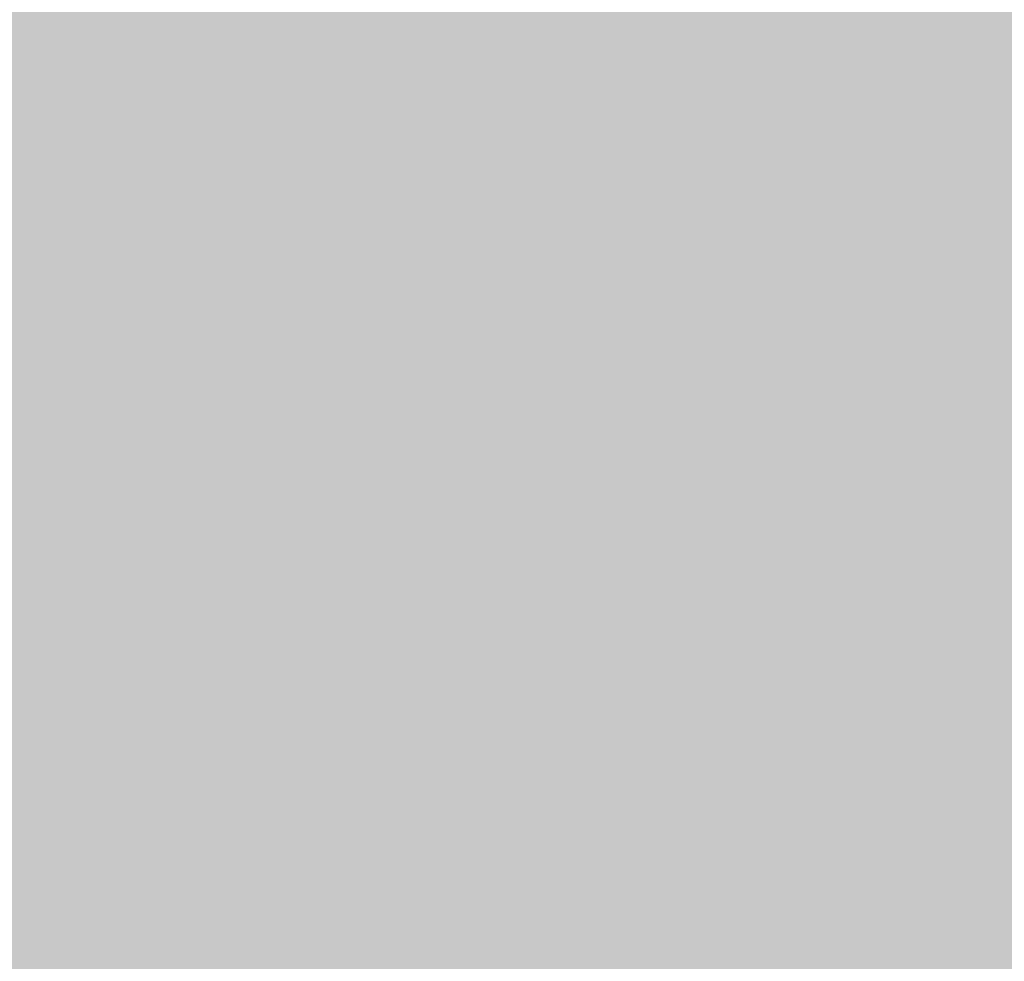
# Model space of a CAD drawing. Units: millimetres. Extents: x 0 to 2267, y 0 to 1823.
# Tile 225 of 256: x 1841.442 to 1842.748, y 1128.399 to 1129.649. Entities that reach past the tile are written whole.
import ezdxf

# ---------------------------------------------------------------- set-up
doc = ezdxf.new("R2010")
doc.units = ezdxf.units.MM
doc.header["$MEASUREMENT"] = 0
doc.layers.add('M-HATC', color=252, linetype='Continuous', lineweight=18)

msp = doc.modelspace()

# ---------------------------------------------------------------- hatches: boundary and pattern name
at = {"layer": 'M-HATC'}
h = msp.add_hatch(color=256, dxfattribs=at)
h.dxf.hatch_style = 1
h.paths.add_polyline_path([(2055.771, 1603.062), (1381.0868, 1603.062), (1381.0868, 1598.062), (2055.771, 1598.062)])
h.paths.add_polyline_path([(2055.771, 1598.062), (1381.0868, 1598.062), (1381.0868, 1593.062), (2055.771, 1593.062)])
h.paths.add_polyline_path([(2051.3074, 1536.7609), (1385.5504, 1536.7609), (1385.5504, 1526.7609), (1387.5504, 1526.7609), (1388.5366, 1525.0528), (1385.3319, 1521.2335), (1385.3319, 1521.2226), (2050.2542, 1522.7491), (2048.3212, 1525.0528), (2049.3074, 1526.7609), (2051.3074, 1526.7609)])
edge = h.paths.add_edge_path()
edge.add_arc((1847.5345, 1379.1492), 135, 222.603061, 222.890851, ccw=False)
edge.add_line((1748.1663, 1287.7656), (1683.0921, 1287.7656))
edge.add_arc((1583.7239, 1379.1492), 135, 317.109149, 317.396939, ccw=False)
edge.add_arc((1678.9686, 1290.6707), 5, 222.8909, 317.1091, ccw=False)
edge.add_arc((1774.2133, 1379.1492), 135, 222.603061, 222.890851, ccw=False)
edge.add_line((1674.8451, 1287.7656), (1609.7709, 1287.7656))
edge.add_arc((1510.4027, 1379.1492), 135, 317.109149, 317.396939, ccw=False)
edge.add_arc((1605.6474, 1290.6707), 5, 222.8909, 317.1091, ccw=False)
edge.add_arc((1700.8921, 1379.1492), 135, 222.603061, 222.890851, ccw=False)
edge.add_line((1601.5239, 1287.7656), (1536.4497, 1287.7656))
edge.add_arc((1437.0815, 1379.1492), 135, 317.109149, 317.396939, ccw=False)
edge.add_arc((1532.3262, 1290.6707), 5, 222.8909, 317.1091, ccw=False)
edge.add_arc((1627.5709, 1379.1492), 135, 222.603061, 222.890851, ccw=False)
edge.add_line((1528.2027, 1287.7656), (1505.9289, 1287.7656))
edge.add_spline(control_points=[(1505.9289, 1287.7656), (1504.2622, 1287.7656), (1504.2622, 1282.7656), (1505.9289, 1282.7656)], knot_values=[0, 0, 0, 0, 5, 5, 5, 5], degree=3, periodic=0)
edge.add_line((1505.9289, 1282.7656), (1930.9289, 1282.7656))
edge.add_spline(control_points=[(1930.9289, 1282.7656), (1932.5956, 1282.7656), (1932.5956, 1287.7656), (1930.9289, 1287.7656)], knot_values=[0, 0, 0, 0, 5, 5, 5, 5], degree=3, periodic=0)
edge.add_line((1930.9289, 1287.7656), (1903.0557, 1287.7656))
edge.add_arc((1803.6875, 1379.1492), 135, 317.109149, 317.396939, ccw=False)
edge.add_arc((1898.9322, 1290.6707), 5, 222.8909, 317.1091, ccw=False)
edge.add_arc((1994.1769, 1379.1492), 135, 222.603061, 222.890851, ccw=False)
edge.add_line((1894.8087, 1287.7656), (1829.7345, 1287.7656))
edge.add_arc((1730.3663, 1379.1492), 135, 317.109149, 317.396939, ccw=False)
edge.add_arc((1825.611, 1290.6707), 5, 222.8909, 317.1091, ccw=False)
edge.add_arc((1920.8557, 1379.1492), 135, 222.603061, 222.890851, ccw=False)
edge.add_line((1821.4875, 1287.7656), (1756.4133, 1287.7656))
edge.add_arc((1657.0451, 1379.1492), 135, 317.109149, 317.396939, ccw=False)
edge.add_arc((1752.2898, 1290.6707), 5, 222.8909, 317.1091, ccw=False)
edge = h.paths.add_edge_path()
edge.add_spline(control_points=[(1843.4289, 1227.2475), (1845.0956, 1227.2475), (1845.0956, 1232.2475), (1843.4289, 1232.2475)], knot_values=[0, 0, 0, 0, 5, 5, 5, 5], degree=3, periodic=0)
edge.add_line((1843.4289, 1232.2475), (1593.4289, 1232.2475))
edge.add_spline(control_points=[(1593.4289, 1232.2475), (1591.7622, 1232.2475), (1591.7622, 1227.2475), (1593.4289, 1227.2475)], knot_values=[0, 0, 0, 0, 5, 5, 5, 5], degree=3, periodic=0)
edge.add_line((1593.4289, 1227.2475), (1843.4289, 1227.2475))
h.paths.add_polyline_path([(1905.9289, 1127.4171), (1530.9289, 1127.4171, 0.414214), (1520.9289, 1117.4171), (1530.9289, 1117.4171), (1915.9289, 1117.4171, 0.414214)])
edge = h.paths.add_edge_path()
edge.add_arc((1397.0858, 1498.4078), 12.7299, 90.78215, 190.87871, ccw=False)
edge.add_line((1396.912, 1511.1365), (1428.0097, 1511.3488))
edge.add_line((1428.0097, 1511.3488), (1433.0097, 1511.3488))
edge.add_line((1433.0097, 1511.3488), (1434.439, 1511.3488))
edge.add_arc((1419.474, 1498.0804), 20, 41.561, 74.08211)
edge.add_line((1424.9592, 1517.3135), (1399.9351, 1517.2561))
edge.add_spline(control_points=[(1399.9307, 1517.2561), (1399.884, 1517.2131), (1399.8328, 1517.1689), (1399.7774, 1517.1236)], knot_values=[11.567499, 11.567499, 11.567499, 11.567499, 11.814249, 11.814249, 11.814249, 11.814249], degree=3, periodic=0)
edge.add_spline(control_points=[(1399.6328, 1517.0099), (1399.5831, 1516.9721), (1399.5307, 1516.9338), (1399.4759, 1516.8947)], knot_values=[11.167718, 11.167718, 11.167718, 11.167718, 11.365188, 11.365188, 11.365188, 11.365188], degree=3, periodic=0)
edge.add_spline(control_points=[(1399.3398, 1516.8001), (1399.1514, 1516.6719), (1398.9384, 1516.5377), (1398.704, 1516.3994)], knot_values=[10.376405, 10.376405, 10.376405, 10.376405, 11.00994, 11.00994, 11.00994, 11.00994], degree=3, periodic=0)
edge.add_spline(control_points=[(1398.6572, 1516.3719), (1398.5789, 1516.326), (1398.4983, 1516.2797), (1398.4155, 1516.2331)], knot_values=[10.125175, 10.125175, 10.125175, 10.125175, 10.334406, 10.334406, 10.334406, 10.334406], degree=3, periodic=0)
edge.add_spline(control_points=[(1398.2642, 1516.1487), (1398.196, 1516.1111), (1398.1263, 1516.0732), (1398.0555, 1516.0351)], knot_values=[9.832246, 9.832246, 9.832246, 9.832246, 9.999658, 9.999658, 9.999658, 9.999658], degree=3, periodic=0)
edge.add_spline(control_points=[(1397.9987, 1516.0048), (1397.7312, 1515.8621), (1397.446, 1515.7171), (1397.1466, 1515.5714)], knot_values=[9.161808, 9.161808, 9.161808, 9.161808, 9.787769, 9.787769, 9.787769, 9.787769], degree=3, periodic=0)
edge.add_spline(control_points=[(1397.1466, 1515.5714), (1396.8418, 1515.423), (1396.5222, 1515.274), (1396.1914, 1515.1262)], knot_values=[8.524455, 8.524455, 8.524455, 8.524455, 9.161808, 9.161808, 9.161808, 9.161808], degree=3, periodic=0)
edge.add_spline(control_points=[(1396.0777, 1515.0756), (1395.9854, 1515.0348), (1395.8922, 1514.994), (1395.7983, 1514.9534)], knot_values=[8.275193, 8.275193, 8.275193, 8.275193, 8.451726, 8.451726, 8.451726, 8.451726], degree=3, periodic=0)
edge.add_spline(control_points=[(1395.6018, 1514.8691), (1395.4997, 1514.8257), (1395.3968, 1514.7824), (1395.2932, 1514.7394)], knot_values=[7.962917, 7.962917, 7.962917, 7.962917, 8.152764, 8.152764, 8.152764, 8.152764], degree=3, periodic=0)
edge.add_spline(control_points=[(1395.2116, 1514.7057), (1394.8278, 1514.5475), (1394.4345, 1514.3929), (1394.0364, 1514.2442)], knot_values=[7.21254, 7.21254, 7.21254, 7.21254, 7.913148, 7.913148, 7.913148, 7.913148], degree=3, periodic=0)
edge.add_spline(control_points=[(1394.0364, 1514.2442), (1393.7076, 1514.1214), (1393.3754, 1514.0027), (1393.0427, 1513.8895)], knot_values=[6.633733, 6.633733, 6.633733, 6.633733, 7.21254, 7.21254, 7.21254, 7.21254], degree=3, periodic=0)
edge.add_spline(control_points=[(1392.8214, 1513.815), (1392.7198, 1513.7812), (1392.6181, 1513.7479), (1392.5166, 1513.7152)], knot_values=[6.328796, 6.328796, 6.328796, 6.328796, 6.505493, 6.505493, 6.505493, 6.505493], degree=3, periodic=0)
edge.add_spline(control_points=[(1392.5166, 1513.7152), (1392.3187, 1513.6515), (1392.1212, 1513.59), (1391.9244, 1513.531)], knot_values=[5.984605, 5.984605, 5.984605, 5.984605, 6.328796, 6.328796, 6.328796, 6.328796], degree=3, periodic=0)
edge.add_spline(control_points=[(1391.7915, 1513.4915), (1391.3122, 1513.3501), (1390.8384, 1513.2239), (1390.3784, 1513.1171)], knot_values=[5.066697, 5.066697, 5.066697, 5.066697, 5.907055, 5.907055, 5.907055, 5.907055], degree=3, periodic=0)
edge.add_spline(control_points=[(1390.3784, 1513.1171), (1390.1797, 1513.071), (1389.9836, 1513.0284), (1389.7907, 1512.9899)], knot_values=[4.70367, 4.70367, 4.70367, 4.70367, 5.066695, 5.066695, 5.066695, 5.066695], degree=3, periodic=0)
edge.add_spline(control_points=[(1389.422, 1512.9204), (1389.2459, 1512.8892), (1389.0729, 1512.8617), (1388.9036, 1512.8381)], knot_values=[4.130571, 4.130571, 4.130571, 4.130571, 4.469816, 4.469816, 4.469816, 4.469816], degree=3, periodic=0)
edge.add_spline(control_points=[(1388.9036, 1512.8381), (1388.591, 1512.7946), (1388.2911, 1512.7644), (1388.0071, 1512.7494)], knot_values=[3.504031, 3.504031, 3.504031, 3.504031, 4.130571, 4.130571, 4.130571, 4.130571], degree=3, periodic=0)
edge.add_spline(control_points=[(1387.9356, 1512.7459), (1387.8538, 1512.7423), (1387.7733, 1512.74), (1387.6944, 1512.739)], knot_values=[3.268866, 3.268866, 3.268866, 3.268866, 3.451164, 3.451164, 3.451164, 3.451164], degree=3, periodic=0)
edge.add_spline(control_points=[(1387.3351, 1512.7443), (1387.2076, 1512.7499), (1387.0847, 1512.7597), (1386.967, 1512.7739)], knot_values=[2.670686, 2.670686, 2.670686, 2.670686, 2.984, 2.984, 2.984, 2.984], degree=3, periodic=0)
edge.add_spline(control_points=[(1386.8327, 1512.7922), (1386.8209, 1512.7941), (1386.8092, 1512.7959), (1386.7975, 1512.7979)], knot_values=[2.516981, 2.516981, 2.516981, 2.516981, 2.549528, 2.549528, 2.549528, 2.549528], degree=3, periodic=0)
edge.add_spline(control_points=[(1386.4526, 1512.8735), (1386.4257, 1512.881), (1386.3993, 1512.889), (1386.3733, 1512.8972)], knot_values=[2.095869, 2.095869, 2.095869, 2.095869, 2.17941, 2.17941, 2.17941, 2.17941], degree=3, periodic=0)
edge.add_spline(control_points=[(1386.0691, 1513.0189), (1386.0634, 1513.0217), (1386.0577, 1513.0246), (1386.052, 1513.0275)], knot_values=[1.72453, 1.72453, 1.72453, 1.72453, 1.745933, 1.745933, 1.745933, 1.745933], degree=3, periodic=0)
edge.add_arc((1399.474, 1498.0804), 20, 131.82432, 180)
edge.add_arc((1630.3336, 1505.5484), 250.9708, 181.705176, 236.427975)
edge.add_arc((1605.3399, 1483.3044), 218.7822, 238.660829, 243.34961)
edge.add_arc((1647.0911, 1510.3592), 262.8986, 183.129836, 237.853442, ccw=False)
h.paths.add_polyline_path([(1406.5369, 1391.9644, 0.149382), (1491.5506, 1296.4418, -0.129517)], flags=17)
edge = h.paths.add_edge_path()
edge.add_arc((2037.3838, 1498.0804), 20, 0, 48.26587)
edge.add_spline(control_points=[(2050.6973, 1513.0052), (2050.6512, 1512.9847), (2050.6034, 1512.9655), (2050.5539, 1512.9477)], knot_values=[1.835652, 1.835652, 1.835652, 1.835652, 2.000781, 2.000781, 2.000781, 2.000781], degree=3, periodic=0)
edge.add_spline(control_points=[(2050.4616, 1512.9166), (2050.479, 1512.9221), (2050.4963, 1512.9277), (2050.5133, 1512.9335)], knot_values=[2.045477, 2.045477, 2.045477, 2.045477, 2.101389, 2.101389, 2.101389, 2.101389], degree=3, periodic=0)
edge.add_spline(control_points=[(2050.129, 1512.8342), (2050.1984, 1512.8473), (2050.2657, 1512.8623), (2050.3308, 1512.8792)], knot_values=[2.237629, 2.237629, 2.237629, 2.237629, 2.435841, 2.435841, 2.435841, 2.435841], degree=3, periodic=0)
edge.add_spline(control_points=[(2050.0946, 1512.8278), (2050.1061, 1512.8299), (2050.1176, 1512.832), (2050.129, 1512.8342)], knot_values=[2.435841, 2.435841, 2.435841, 2.435841, 2.468321, 2.468321, 2.468321, 2.468321], degree=3, periodic=0)
edge.add_spline(control_points=[(2049.7843, 1512.7851), (2049.8552, 1512.7922), (2049.9243, 1512.8008), (2049.9917, 1512.8109)], knot_values=[2.563852, 2.563852, 2.563852, 2.563852, 2.748541, 2.748541, 2.748541, 2.748541], degree=3, periodic=0)
edge.add_spline(control_points=[(2049.4052, 1512.7617), (2049.5364, 1512.7653), (2049.6629, 1512.773), (2049.7843, 1512.7851)], knot_values=[2.748541, 2.748541, 2.748541, 2.748541, 3.064882, 3.064882, 3.064882, 3.064882], degree=3, periodic=0)
edge.add_spline(control_points=[(2049.1698, 1512.7597), (2049.2336, 1512.7591), (2049.2965, 1512.7594), (2049.3584, 1512.7606)], knot_values=[3.102309, 3.102309, 3.102309, 3.102309, 3.2503, 3.2503, 3.2503, 3.2503], degree=3, periodic=0)
edge.add_spline(control_points=[(2048.8573, 1512.7691), (2048.9638, 1512.7638), (2049.068, 1512.7606), (2049.1698, 1512.7597)], knot_values=[3.2503, 3.2503, 3.2503, 3.2503, 3.486069, 3.486069, 3.486069, 3.486069], degree=3, periodic=0)
edge.add_spline(control_points=[(2048.6924, 1512.7789), (2048.3729, 1512.8009), (2048.0345, 1512.8411), (2047.6817, 1512.897)], knot_values=[3.606429, 3.606429, 3.606429, 3.606429, 4.2989, 4.2989, 4.2989, 4.2989], degree=3, periodic=0)
edge.add_spline(control_points=[(2047.6817, 1512.897), (2047.5458, 1512.9185), (2047.4077, 1512.9424), (2047.2678, 1512.9685)], knot_values=[4.2989, 4.2989, 4.2989, 4.2989, 4.565769, 4.565769, 4.565769, 4.565769], degree=3, periodic=0)
edge.add_spline(control_points=[(2047.2678, 1512.9685), (2047.1449, 1512.9914), (2047.0207, 1513.016), (2046.8951, 1513.0422)], knot_values=[4.565769, 4.565769, 4.565769, 4.565769, 4.799971, 4.799971, 4.799971, 4.799971], degree=3, periodic=0)
edge.add_spline(control_points=[(2046.8951, 1513.0422), (2046.5286, 1513.1188), (2046.1513, 1513.209), (2045.7676, 1513.3107)], knot_values=[4.799971, 4.799971, 4.799971, 4.799971, 5.483718, 5.483718, 5.483718, 5.483718], degree=3, periodic=0)
edge.add_spline(control_points=[(2045.7676, 1513.3107), (2045.3724, 1513.4154), (2044.9704, 1513.5322), (2044.5662, 1513.6588)], knot_values=[5.483718, 5.483718, 5.483718, 5.483718, 6.187866, 6.187866, 6.187866, 6.187866], degree=3, periodic=0)
edge.add_spline(control_points=[(2044.5662, 1513.6588), (2044.4149, 1513.7061), (2044.2633, 1513.7549), (2044.1116, 1513.8048)], knot_values=[6.187866, 6.187866, 6.187866, 6.187866, 6.451551, 6.451551, 6.451551, 6.451551], degree=3, periodic=0)
edge.add_spline(control_points=[(2044.1116, 1513.8048), (2043.9967, 1513.8427), (2043.8817, 1513.8813), (2043.7668, 1513.9205)], knot_values=[6.451551, 6.451551, 6.451551, 6.451551, 6.651434, 6.651434, 6.651434, 6.651434], degree=3, periodic=0)
edge.add_spline(control_points=[(2043.7668, 1513.9205), (2043.3716, 1514.0554), (2042.9774, 1514.1979), (2042.5886, 1514.3458)], knot_values=[6.651434, 6.651434, 6.651434, 6.651434, 7.338879, 7.338879, 7.338879, 7.338879], degree=3, periodic=0)
edge.add_spline(control_points=[(2042.5886, 1514.3458), (2042.1643, 1514.5071), (2041.7465, 1514.6749), (2041.3409, 1514.846)], knot_values=[7.338879, 7.338879, 7.338879, 7.338879, 8.089209, 8.089209, 8.089209, 8.089209], degree=3, periodic=0)
edge.add_spline(control_points=[(2041.3409, 1514.846), (2041.1028, 1514.9465), (2040.869, 1515.0481), (2040.6405, 1515.1502)], knot_values=[8.089209, 8.089209, 8.089209, 8.089209, 8.529587, 8.529587, 8.529587, 8.529587], degree=3, periodic=0)
edge.add_spline(control_points=[(2040.51, 1515.2089), (2040.0824, 1515.4022), (2039.6747, 1515.5971), (2039.295, 1515.7894)], knot_values=[8.613818, 8.613818, 8.613818, 8.613818, 9.44571, 9.44571, 9.44571, 9.44571], degree=3, periodic=0)
edge.add_spline(control_points=[(2039.295, 1515.7894), (2039.0618, 1515.9075), (2038.8391, 1516.0246), (2038.6288, 1516.1398)], knot_values=[9.44571, 9.44571, 9.44571, 9.44571, 9.956404, 9.956404, 9.956404, 9.956404], degree=3, periodic=0)
edge.add_spline(control_points=[(2038.6288, 1516.1398), (2038.5187, 1516.2001), (2038.4121, 1516.2598), (2038.309, 1516.3189)], knot_values=[9.956404, 9.956404, 9.956404, 9.956404, 10.223542, 10.223542, 10.223542, 10.223542], degree=3, periodic=0)
edge.add_spline(control_points=[(2038.309, 1516.3189), (2038.2138, 1516.3735), (2038.1216, 1516.4276), (2038.0328, 1516.481)], knot_values=[10.223542, 10.223542, 10.223542, 10.223542, 10.47051, 10.47051, 10.47051, 10.47051], degree=3, periodic=0)
edge.add_spline(control_points=[(2038.0328, 1516.481), (2037.7855, 1516.6296), (2037.5639, 1516.773), (2037.3722, 1516.909)], knot_values=[10.47051, 10.47051, 10.47051, 10.47051, 11.15767, 11.15767, 11.15767, 11.15767], degree=3, periodic=0)
edge.add_spline(control_points=[(2037.3722, 1516.909), (2037.2789, 1516.9752), (2037.1927, 1517.0396), (2037.1142, 1517.102)], knot_values=[11.15767, 11.15767, 11.15767, 11.15767, 11.49227, 11.49227, 11.49227, 11.49227], degree=3, periodic=0)
edge.add_spline(control_points=[(2036.8564, 1517.3259), (2036.9148, 1517.2692), (2036.9814, 1517.2103), (2037.0557, 1517.1492)], knot_values=[11.577341, 11.577341, 11.577341, 11.577341, 11.91035, 11.91035, 11.91035, 11.91035], degree=3, periodic=0)
edge.add_spline(control_points=[(2036.8074, 1517.3748), (2036.823, 1517.3587), (2036.8393, 1517.3424), (2036.8564, 1517.3259)], knot_values=[11.91035, 11.91035, 11.91035, 11.91035, 12.007402, 12.007402, 12.007402, 12.007402], degree=3, periodic=0)
edge.add_spline(control_points=[(2036.7017, 1517.494), (2036.7104, 1517.483), (2036.7196, 1517.4719), (2036.7291, 1517.4606)], knot_values=[12.184155, 12.184155, 12.184155, 12.184155, 12.255409, 12.255409, 12.255409, 12.255409], degree=3, periodic=0)
edge.add_spline(control_points=[(2036.6159, 1517.6205), (2036.62, 1517.613), (2036.6243, 1517.6055), (2036.6289, 1517.5979)], knot_values=[12.487913, 12.487913, 12.487913, 12.487913, 12.541035, 12.541035, 12.541035, 12.541035], degree=3, periodic=0)
edge.add_spline(control_points=[(2036.5635, 1517.786), (2036.5637, 1517.7794), (2036.5642, 1517.7726), (2036.565, 1517.7658)], knot_values=[12.911761, 12.911761, 12.911761, 12.911761, 12.968286, 12.968286, 12.968286, 12.968286], degree=3, periodic=0)
edge.add_spline(control_points=[(2036.6166, 1517.9304), (2036.6125, 1517.9259), (2036.6086, 1517.9212), (2036.6049, 1517.9165)], knot_values=[13.382527, 13.382527, 13.382527, 13.382527, 13.433791, 13.433791, 13.433791, 13.433791], degree=3, periodic=0)
edge.add_spline(control_points=[(2036.749, 1518.017), (2036.7361, 1518.0116), (2036.7239, 1518.006), (2036.7124, 1518.0002)], knot_values=[13.726299, 13.726299, 13.726299, 13.726299, 13.809928, 13.809928, 13.809928, 13.809928], degree=3, periodic=0)
edge.add_spline(control_points=[(2036.8604, 1518.0528), (2036.8386, 1518.0474), (2036.8181, 1518.0416), (2036.7988, 1518.0353)], knot_values=[13.910887, 13.910887, 13.910887, 13.910887, 14.02153, 14.02153, 14.02153, 14.02153], degree=3, periodic=0)
edge.add_line((2036.9639, 1518.0804), (2032.3838, 1518.0804))
edge.add_line((2032.3838, 1518.0804), (2027.3838, 1518.0804))
edge.add_line((2027.3838, 1518.0804), (2022.3838, 1518.0804))
edge.add_line((2022.3838, 1518.0804), (2017.3838, 1518.0804))
edge.add_arc((2017.3838, 1498.0804), 20, 90, 138.439)
edge.add_line((2002.4188, 1511.3488), (2003.8481, 1511.3488))
edge.add_line((2003.8481, 1511.3488), (2008.8481, 1511.3488))
edge.add_line((2008.8481, 1511.3488), (2039.772, 1511.1377))
edge.add_arc((2039.772, 1498.4078), 12.7299, -10.87871, 90, ccw=False)
edge.add_arc((1789.7668, 1510.3592), 262.8986, 302.146558, 356.870164, ccw=False)
edge.add_arc((1831.5179, 1483.3044), 218.7822, 296.65039, 301.339171)
edge.add_arc((1806.5242, 1505.5484), 250.9708, 303.572025, 358.294824)
h.paths.add_polyline_path([(2030.321, 1391.9644, -0.129517), (1945.3072, 1296.4418, 0.149382)], flags=17)
edge = h.paths.add_edge_path()
edge.add_spline(control_points=[(2037.2464, 1518.0821), (2037.2898, 1518.081), (2037.3355, 1518.0804), (2037.3838, 1518.0804)], knot_values=[0.000012, 0.000012, 0.000012, 0.000012, 0.144754, 0.144754, 0.144754, 0.144754], degree=3, periodic=0)
edge.add_line((2037.3357, 1518.0804), (2037.0096, 1518.0804))
edge.add_spline(control_points=[(2037.0096, 1518.0804), (2036.9822, 1518.0768), (2036.956, 1518.0727), (2036.9312, 1518.0681)], knot_values=[14.13465, 14.13465, 14.13465, 14.13465, 14.247197, 14.247197, 14.247197, 14.247197], degree=3, periodic=0)
edge.add_spline(control_points=[(2036.9312, 1518.0681), (2036.9276, 1518.0674), (2036.9241, 1518.0667), (2036.9205, 1518.0661)], knot_values=[14.118315, 14.118315, 14.118315, 14.118315, 14.13465, 14.13465, 14.13465, 14.13465], degree=3, periodic=0)
edge.add_spline(control_points=[(2036.9205, 1518.0661), (2036.9118, 1518.0644), (2036.9032, 1518.0626), (2036.8948, 1518.0608)], knot_values=[14.078086, 14.078086, 14.078086, 14.078086, 14.118315, 14.118315, 14.118315, 14.118315], degree=3, periodic=0)
edge.add_spline(control_points=[(2036.8948, 1518.0608), (2036.883, 1518.0583), (2036.8716, 1518.0556), (2036.8604, 1518.0528)], knot_values=[14.02153, 14.02153, 14.02153, 14.02153, 14.078086, 14.078086, 14.078086, 14.078086], degree=3, periodic=0)
edge.add_spline(control_points=[(2036.8604, 1518.0528), (2036.8386, 1518.0474), (2036.8181, 1518.0416), (2036.7988, 1518.0353)], knot_values=[13.910887, 13.910887, 13.910887, 13.910887, 14.02153, 14.02153, 14.02153, 14.02153], degree=3, periodic=0)
edge.add_spline(control_points=[(2036.7988, 1518.0353), (2036.7981, 1518.035), (2036.7974, 1518.0348), (2036.7967, 1518.0346)], knot_values=[13.906906, 13.906906, 13.906906, 13.906906, 13.910887, 13.910887, 13.910887, 13.910887], degree=3, periodic=0)
edge.add_spline(control_points=[(2036.7967, 1518.0346), (2036.7882, 1518.0318), (2036.7799, 1518.0289), (2036.7719, 1518.0259)], knot_values=[13.857826, 13.857826, 13.857826, 13.857826, 13.906906, 13.906906, 13.906906, 13.906906], degree=3, periodic=0)
edge.add_spline(control_points=[(2036.7719, 1518.0259), (2036.764, 1518.023), (2036.7564, 1518.02), (2036.749, 1518.017)], knot_values=[13.809928, 13.809928, 13.809928, 13.809928, 13.857826, 13.857826, 13.857826, 13.857826], degree=3, periodic=0)
edge.add_spline(control_points=[(2036.749, 1518.017), (2036.7361, 1518.0116), (2036.7239, 1518.006), (2036.7124, 1518.0002)], knot_values=[13.726299, 13.726299, 13.726299, 13.726299, 13.809928, 13.809928, 13.809928, 13.809928], degree=3, periodic=0)
edge.add_spline(control_points=[(2036.7124, 1518.0002), (2036.7121, 1518), (2036.7118, 1517.9999), (2036.7115, 1517.9997)], knot_values=[13.723993, 13.723993, 13.723993, 13.723993, 13.726299, 13.726299, 13.726299, 13.726299], degree=3, periodic=0)
edge.add_spline(control_points=[(2036.7115, 1517.9997), (2036.7063, 1517.9971), (2036.7013, 1517.9944), (2036.6965, 1517.9917)], knot_values=[13.686536, 13.686536, 13.686536, 13.686536, 13.723993, 13.723993, 13.723993, 13.723993], degree=3, periodic=0)
edge.add_spline(control_points=[(2036.6965, 1517.9917), (2036.6919, 1517.9891), (2036.6874, 1517.9865), (2036.6831, 1517.9839)], knot_values=[13.651251, 13.651251, 13.651251, 13.651251, 13.686536, 13.686536, 13.686536, 13.686536], degree=3, periodic=0)
edge.add_spline(control_points=[(2036.6831, 1517.9839), (2036.6764, 1517.9798), (2036.67, 1517.9757), (2036.6639, 1517.9714)], knot_values=[13.596804, 13.596804, 13.596804, 13.596804, 13.651251, 13.651251, 13.651251, 13.651251], degree=3, periodic=0)
edge.add_spline(control_points=[(2036.6639, 1517.9714), (2036.6636, 1517.9712), (2036.6633, 1517.9709), (2036.6629, 1517.9707)], knot_values=[13.593956, 13.593956, 13.593956, 13.593956, 13.596804, 13.596804, 13.596804, 13.596804], degree=3, periodic=0)
edge.add_spline(control_points=[(2036.6629, 1517.9707), (2036.6603, 1517.9689), (2036.6577, 1517.967), (2036.6552, 1517.9651)], knot_values=[13.570322, 13.570322, 13.570322, 13.570322, 13.593956, 13.593956, 13.593956, 13.593956], degree=3, periodic=0)
edge.add_spline(control_points=[(2036.6552, 1517.9651), (2036.6525, 1517.9631), (2036.6499, 1517.9611), (2036.6474, 1517.9591)], knot_values=[13.545477, 13.545477, 13.545477, 13.545477, 13.570322, 13.570322, 13.570322, 13.570322], degree=3, periodic=0)
edge.add_spline(control_points=[(2036.6474, 1517.9591), (2036.6472, 1517.9589), (2036.6471, 1517.9588), (2036.6469, 1517.9587)], knot_values=[13.543931, 13.543931, 13.543931, 13.543931, 13.545477, 13.545477, 13.545477, 13.545477], degree=3, periodic=0)
edge.add_spline(control_points=[(2036.6469, 1517.9587), (2036.6412, 1517.9541), (2036.6358, 1517.9494), (2036.6307, 1517.9447)], knot_values=[13.488237, 13.488237, 13.488237, 13.488237, 13.543931, 13.543931, 13.543931, 13.543931], degree=3, periodic=0)
edge.add_spline(control_points=[(2036.6307, 1517.9447), (2036.6282, 1517.9423), (2036.6257, 1517.9399), (2036.6233, 1517.9374)], knot_values=[13.460307, 13.460307, 13.460307, 13.460307, 13.488237, 13.488237, 13.488237, 13.488237], degree=3, periodic=0)
edge.add_spline(control_points=[(2036.6233, 1517.9374), (2036.6215, 1517.9356), (2036.6198, 1517.9338), (2036.6181, 1517.932)], knot_values=[13.439712, 13.439712, 13.439712, 13.439712, 13.460307, 13.460307, 13.460307, 13.460307], degree=3, periodic=0)
edge.add_spline(control_points=[(2036.6181, 1517.932), (2036.6176, 1517.9315), (2036.6171, 1517.9309), (2036.6166, 1517.9304)], knot_values=[13.433791, 13.433791, 13.433791, 13.433791, 13.439712, 13.439712, 13.439712, 13.439712], degree=3, periodic=0)
edge.add_spline(control_points=[(2036.6166, 1517.9304), (2036.6125, 1517.9259), (2036.6086, 1517.9212), (2036.6049, 1517.9165)], knot_values=[13.382527, 13.382527, 13.382527, 13.382527, 13.433791, 13.433791, 13.433791, 13.433791], degree=3, periodic=0)
edge.add_spline(control_points=[(2036.6049, 1517.9165), (2036.6026, 1517.9135), (2036.6004, 1517.9104), (2036.5982, 1517.9074)], knot_values=[13.350017, 13.350017, 13.350017, 13.350017, 13.382527, 13.382527, 13.382527, 13.382527], degree=3, periodic=0)
edge.add_spline(control_points=[(2036.5982, 1517.9074), (2036.5972, 1517.9059), (2036.5962, 1517.9043), (2036.5952, 1517.9028)], knot_values=[13.333922, 13.333922, 13.333922, 13.333922, 13.350017, 13.350017, 13.350017, 13.350017], degree=3, periodic=0)
edge.add_spline(control_points=[(2036.5952, 1517.9028), (2036.5945, 1517.9018), (2036.5939, 1517.9009), (2036.5933, 1517.8999)], knot_values=[13.323828, 13.323828, 13.323828, 13.323828, 13.333922, 13.333922, 13.333922, 13.333922], degree=3, periodic=0)
edge.add_spline(control_points=[(2036.5933, 1517.8999), (2036.5905, 1517.8955), (2036.5879, 1517.8909), (2036.5855, 1517.8864)], knot_values=[13.277545, 13.277545, 13.277545, 13.277545, 13.323828, 13.323828, 13.323828, 13.323828], degree=3, periodic=0)
edge.add_spline(control_points=[(2036.5855, 1517.8864), (2036.5836, 1517.8827), (2036.5817, 1517.8789), (2036.5801, 1517.8751)], knot_values=[13.240119, 13.240119, 13.240119, 13.240119, 13.277545, 13.277545, 13.277545, 13.277545], degree=3, periodic=0)
edge.add_spline(control_points=[(2036.5801, 1517.8751), (2036.5795, 1517.8739), (2036.579, 1517.8727), (2036.5785, 1517.8715)], knot_values=[13.228211, 13.228211, 13.228211, 13.228211, 13.240119, 13.240119, 13.240119, 13.240119], degree=3, periodic=0)
edge.add_spline(control_points=[(2036.5785, 1517.8715), (2036.578, 1517.8702), (2036.5774, 1517.869), (2036.5769, 1517.8677)], knot_values=[13.215717, 13.215717, 13.215717, 13.215717, 13.228211, 13.228211, 13.228211, 13.228211], degree=3, periodic=0)
edge.add_spline(control_points=[(2036.5769, 1517.8677), (2036.5755, 1517.864), (2036.5741, 1517.8603), (2036.5729, 1517.8565)], knot_values=[13.179847, 13.179847, 13.179847, 13.179847, 13.215717, 13.215717, 13.215717, 13.215717], degree=3, periodic=0)
edge.add_spline(control_points=[(2036.5729, 1517.8565), (2036.5713, 1517.8515), (2036.5699, 1517.8464), (2036.5687, 1517.8413)], knot_values=[13.132017, 13.132017, 13.132017, 13.132017, 13.179847, 13.179847, 13.179847, 13.179847], degree=3, periodic=0)
edge.add_spline(control_points=[(2036.5687, 1517.8413), (2036.5684, 1517.8402), (2036.5682, 1517.8392), (2036.568, 1517.8382)], knot_values=[13.122482, 13.122482, 13.122482, 13.122482, 13.132017, 13.132017, 13.132017, 13.132017], degree=3, periodic=0)
edge.add_spline(control_points=[(2036.568, 1517.8382), (2036.5676, 1517.8363), (2036.5672, 1517.8345), (2036.5669, 1517.8327)], knot_values=[13.105592, 13.105592, 13.105592, 13.105592, 13.122482, 13.122482, 13.122482, 13.122482], degree=3, periodic=0)
edge.add_spline(control_points=[(2036.5669, 1517.8327), (2036.5662, 1517.8292), (2036.5657, 1517.8257), (2036.5652, 1517.8222)], knot_values=[13.074063, 13.074063, 13.074063, 13.074063, 13.105592, 13.105592, 13.105592, 13.105592], degree=3, periodic=0)
edge.add_spline(control_points=[(2036.5652, 1517.8222), (2036.5652, 1517.8222), (2036.5652, 1517.8222), (2036.5652, 1517.8222)], knot_values=[13.074043, 13.074043, 13.074043, 13.074043, 13.074063, 13.074063, 13.074063, 13.074063], degree=3, periodic=0)
edge.add_spline(control_points=[(2036.5652, 1517.8222), (2036.5644, 1517.8164), (2036.5639, 1517.8106), (2036.5636, 1517.8046)], knot_values=[13.021884, 13.021884, 13.021884, 13.021884, 13.074043, 13.074043, 13.074043, 13.074043], degree=3, periodic=0)
edge.add_spline(control_points=[(2036.5636, 1517.8046), (2036.5636, 1517.804), (2036.5636, 1517.8034), (2036.5635, 1517.8028)], knot_values=[13.01674, 13.01674, 13.01674, 13.01674, 13.021884, 13.021884, 13.021884, 13.021884], degree=3, periodic=0)
edge.add_spline(control_points=[(2036.5635, 1517.8028), (2036.5634, 1517.8005), (2036.5634, 1517.7982), (2036.5634, 1517.7958)], knot_values=[12.996438, 12.996438, 12.996438, 12.996438, 13.01674, 13.01674, 13.01674, 13.01674], degree=3, periodic=0)
edge.add_spline(control_points=[(2036.5634, 1517.7958), (2036.5633, 1517.7926), (2036.5634, 1517.7893), (2036.5635, 1517.786)], knot_values=[12.968286, 12.968286, 12.968286, 12.968286, 12.996438, 12.996438, 12.996438, 12.996438], degree=3, periodic=0)
edge.add_spline(control_points=[(2036.5635, 1517.786), (2036.5637, 1517.7794), (2036.5642, 1517.7726), (2036.565, 1517.7658)], knot_values=[12.911761, 12.911761, 12.911761, 12.911761, 12.968286, 12.968286, 12.968286, 12.968286], degree=3, periodic=0)
edge.add_spline(control_points=[(2036.565, 1517.7658), (2036.565, 1517.7657), (2036.565, 1517.7656), (2036.565, 1517.7656)], knot_values=[12.911017, 12.911017, 12.911017, 12.911017, 12.911761, 12.911761, 12.911761, 12.911761], degree=3, periodic=0)
edge.add_spline(control_points=[(2036.565, 1517.7656), (2036.5654, 1517.7625), (2036.5658, 1517.7593), (2036.5663, 1517.7562)], knot_values=[12.88528, 12.88528, 12.88528, 12.88528, 12.911017, 12.911017, 12.911017, 12.911017], degree=3, periodic=0)
edge.add_spline(control_points=[(2036.5663, 1517.7562), (2036.5667, 1517.7534), (2036.5672, 1517.7506), (2036.5677, 1517.7478)], knot_values=[12.862519, 12.862519, 12.862519, 12.862519, 12.88528, 12.88528, 12.88528, 12.88528], degree=3, periodic=0)
edge.add_spline(control_points=[(2036.5677, 1517.7478), (2036.5678, 1517.7474), (2036.5679, 1517.7469), (2036.568, 1517.7465)], knot_values=[12.858885, 12.858885, 12.858885, 12.858885, 12.862519, 12.862519, 12.862519, 12.862519], degree=3, periodic=0)
edge.add_spline(control_points=[(2036.568, 1517.7465), (2036.5692, 1517.7399), (2036.5707, 1517.7332), (2036.5724, 1517.7264)], knot_values=[12.8053, 12.8053, 12.8053, 12.8053, 12.858885, 12.858885, 12.858885, 12.858885], degree=3, periodic=0)
edge.add_spline(control_points=[(2036.5724, 1517.7264), (2036.5734, 1517.7226), (2036.5745, 1517.7187), (2036.5756, 1517.7149)], knot_values=[12.775176, 12.775176, 12.775176, 12.775176, 12.8053, 12.8053, 12.8053, 12.8053], degree=3, periodic=0)
edge.add_spline(control_points=[(2036.5756, 1517.7149), (2036.5763, 1517.7125), (2036.577, 1517.7102), (2036.5778, 1517.7078)], knot_values=[12.756759, 12.756759, 12.756759, 12.756759, 12.775176, 12.775176, 12.775176, 12.775176], degree=3, periodic=0)
edge.add_spline(control_points=[(2036.5778, 1517.7078), (2036.5781, 1517.7067), (2036.5784, 1517.7057), (2036.5787, 1517.7047)], knot_values=[12.748742, 12.748742, 12.748742, 12.748742, 12.756759, 12.756759, 12.756759, 12.756759], degree=3, periodic=0)
edge.add_spline(control_points=[(2036.5787, 1517.7047), (2036.5808, 1517.6983), (2036.5831, 1517.6919), (2036.5856, 1517.6854)], knot_values=[12.69959, 12.69959, 12.69959, 12.69959, 12.748742, 12.748742, 12.748742, 12.748742], degree=3, periodic=0)
edge.add_spline(control_points=[(2036.5856, 1517.6854), (2036.5876, 1517.68), (2036.5898, 1517.6746), (2036.5921, 1517.6692)], knot_values=[12.659038, 12.659038, 12.659038, 12.659038, 12.69959, 12.69959, 12.69959, 12.69959], degree=3, periodic=0)
edge.add_spline(control_points=[(2036.5921, 1517.6692), (2036.594, 1517.6648), (2036.5959, 1517.6605), (2036.5979, 1517.6561)], knot_values=[12.626806, 12.626806, 12.626806, 12.626806, 12.659038, 12.659038, 12.659038, 12.659038], degree=3, periodic=0)
edge.add_spline(control_points=[(2036.5979, 1517.6561), (2036.5984, 1517.6551), (2036.5989, 1517.6541), (2036.5993, 1517.6531)], knot_values=[12.619394, 12.619394, 12.619394, 12.619394, 12.626806, 12.626806, 12.626806, 12.626806], degree=3, periodic=0)
edge.add_spline(control_points=[(2036.5993, 1517.6531), (2036.6043, 1517.6424), (2036.6099, 1517.6315), (2036.6159, 1517.6205)], knot_values=[12.541039, 12.541039, 12.541039, 12.541039, 12.619394, 12.619394, 12.619394, 12.619394], degree=3, periodic=0)
edge.add_spline(control_points=[(2036.6159, 1517.6205), (2036.6159, 1517.6205), (2036.6159, 1517.6205), (2036.6159, 1517.6205)], knot_values=[12.541035, 12.541035, 12.541035, 12.541035, 12.541039, 12.541039, 12.541039, 12.541039], degree=3, periodic=0)
edge.add_spline(control_points=[(2036.6159, 1517.6205), (2036.62, 1517.613), (2036.6243, 1517.6055), (2036.6289, 1517.5979)], knot_values=[12.487913, 12.487913, 12.487913, 12.487913, 12.541035, 12.541035, 12.541035, 12.541035], degree=3, periodic=0)
edge.add_spline(control_points=[(2036.6289, 1517.5979), (2036.6326, 1517.5916), (2036.6365, 1517.5853), (2036.6406, 1517.5789)], knot_values=[12.443982, 12.443982, 12.443982, 12.443982, 12.487913, 12.487913, 12.487913, 12.487913], degree=3, periodic=0)
edge.add_spline(control_points=[(2036.6406, 1517.5789), (2036.6414, 1517.5776), (2036.6423, 1517.5763), (2036.6431, 1517.5749)], knot_values=[12.434996, 12.434996, 12.434996, 12.434996, 12.443982, 12.443982, 12.443982, 12.443982], degree=3, periodic=0)
edge.add_spline(control_points=[(2036.6431, 1517.5749), (2036.6531, 1517.5596), (2036.6639, 1517.5439), (2036.6756, 1517.528)], knot_values=[12.329647, 12.329647, 12.329647, 12.329647, 12.434996, 12.434996, 12.434996, 12.434996], degree=3, periodic=0)
edge.add_spline(control_points=[(2036.6756, 1517.528), (2036.6839, 1517.5168), (2036.6925, 1517.5055), (2036.7017, 1517.494)], knot_values=[12.255409, 12.255409, 12.255409, 12.255409, 12.329647, 12.329647, 12.329647, 12.329647], degree=3, periodic=0)
edge.add_spline(control_points=[(2036.7017, 1517.494), (2036.7104, 1517.483), (2036.7196, 1517.4719), (2036.7291, 1517.4606)], knot_values=[12.184155, 12.184155, 12.184155, 12.184155, 12.255409, 12.255409, 12.255409, 12.255409], degree=3, periodic=0)
edge.add_spline(control_points=[(2036.7291, 1517.4606), (2036.7436, 1517.4435), (2036.759, 1517.4262), (2036.7753, 1517.4085)], knot_values=[12.075961, 12.075961, 12.075961, 12.075961, 12.184155, 12.184155, 12.184155, 12.184155], degree=3, periodic=0)
edge.add_spline(control_points=[(2036.7753, 1517.4085), (2036.7763, 1517.4075), (2036.7773, 1517.4064), (2036.7783, 1517.4054)], knot_values=[12.069502, 12.069502, 12.069502, 12.069502, 12.075961, 12.075961, 12.075961, 12.075961], degree=3, periodic=0)
edge.add_spline(control_points=[(2036.7783, 1517.4054), (2036.7877, 1517.3953), (2036.7974, 1517.385), (2036.8074, 1517.3748)], knot_values=[12.007402, 12.007402, 12.007402, 12.007402, 12.069502, 12.069502, 12.069502, 12.069502], degree=3, periodic=0)
edge.add_spline(control_points=[(2036.8074, 1517.3748), (2036.823, 1517.3587), (2036.8393, 1517.3424), (2036.8564, 1517.3259)], knot_values=[11.91035, 11.91035, 11.91035, 11.91035, 12.007402, 12.007402, 12.007402, 12.007402], degree=3, periodic=0)
edge.add_spline(control_points=[(2036.8564, 1517.3259), (2036.9148, 1517.2692), (2036.9814, 1517.2103), (2037.0557, 1517.1492)], knot_values=[11.577341, 11.577341, 11.577341, 11.577341, 11.91035, 11.91035, 11.91035, 11.91035], degree=3, periodic=0)
edge.add_spline(control_points=[(2037.0557, 1517.1492), (2037.0747, 1517.1336), (2037.0942, 1517.1179), (2037.1142, 1517.102)], knot_values=[11.49227, 11.49227, 11.49227, 11.49227, 11.577341, 11.577341, 11.577341, 11.577341], degree=3, periodic=0)
edge.add_spline(control_points=[(2037.1142, 1517.102), (2037.1927, 1517.0396), (2037.2789, 1516.9752), (2037.3722, 1516.909)], knot_values=[11.15767, 11.15767, 11.15767, 11.15767, 11.49227, 11.49227, 11.49227, 11.49227], degree=3, periodic=0)
edge.add_spline(control_points=[(2037.3722, 1516.909), (2037.5639, 1516.773), (2037.7855, 1516.6296), (2038.0328, 1516.481)], knot_values=[10.47051, 10.47051, 10.47051, 10.47051, 11.15767, 11.15767, 11.15767, 11.15767], degree=3, periodic=0)
edge.add_spline(control_points=[(2038.0328, 1516.481), (2038.1216, 1516.4276), (2038.2138, 1516.3735), (2038.309, 1516.3189)], knot_values=[10.223542, 10.223542, 10.223542, 10.223542, 10.47051, 10.47051, 10.47051, 10.47051], degree=3, periodic=0)
edge.add_spline(control_points=[(2038.309, 1516.3189), (2038.4121, 1516.2598), (2038.5187, 1516.2001), (2038.6288, 1516.1398)], knot_values=[9.956404, 9.956404, 9.956404, 9.956404, 10.223542, 10.223542, 10.223542, 10.223542], degree=3, periodic=0)
edge.add_spline(control_points=[(2038.6288, 1516.1398), (2038.8391, 1516.0246), (2039.0618, 1515.9075), (2039.295, 1515.7894)], knot_values=[9.44571, 9.44571, 9.44571, 9.44571, 9.956404, 9.956404, 9.956404, 9.956404], degree=3, periodic=0)
edge.add_spline(control_points=[(2039.295, 1515.7894), (2039.6747, 1515.5971), (2040.0824, 1515.4022), (2040.51, 1515.2089)], knot_values=[8.613818, 8.613818, 8.613818, 8.613818, 9.44571, 9.44571, 9.44571, 9.44571], degree=3, periodic=0)
edge.add_spline(control_points=[(2040.51, 1515.2089), (2040.5533, 1515.1893), (2040.5968, 1515.1697), (2040.6405, 1515.1502)], knot_values=[8.529587, 8.529587, 8.529587, 8.529587, 8.613818, 8.613818, 8.613818, 8.613818], degree=3, periodic=0)
edge.add_spline(control_points=[(2040.6405, 1515.1502), (2040.869, 1515.0481), (2041.1028, 1514.9465), (2041.3409, 1514.846)], knot_values=[8.089209, 8.089209, 8.089209, 8.089209, 8.529587, 8.529587, 8.529587, 8.529587], degree=3, periodic=0)
edge.add_spline(control_points=[(2041.3409, 1514.846), (2041.7465, 1514.6749), (2042.1643, 1514.5071), (2042.5886, 1514.3458)], knot_values=[7.338879, 7.338879, 7.338879, 7.338879, 8.089209, 8.089209, 8.089209, 8.089209], degree=3, periodic=0)
edge.add_spline(control_points=[(2042.5886, 1514.3458), (2042.9774, 1514.1979), (2043.3716, 1514.0554), (2043.7668, 1513.9205)], knot_values=[6.651434, 6.651434, 6.651434, 6.651434, 7.338879, 7.338879, 7.338879, 7.338879], degree=3, periodic=0)
edge.add_spline(control_points=[(2043.7668, 1513.9205), (2043.8817, 1513.8813), (2043.9967, 1513.8427), (2044.1116, 1513.8048)], knot_values=[6.451551, 6.451551, 6.451551, 6.451551, 6.651434, 6.651434, 6.651434, 6.651434], degree=3, periodic=0)
edge.add_spline(control_points=[(2044.1116, 1513.8048), (2044.2633, 1513.7549), (2044.4149, 1513.7061), (2044.5662, 1513.6588)], knot_values=[6.187866, 6.187866, 6.187866, 6.187866, 6.451551, 6.451551, 6.451551, 6.451551], degree=3, periodic=0)
edge.add_spline(control_points=[(2044.5662, 1513.6588), (2044.9704, 1513.5322), (2045.3724, 1513.4154), (2045.7676, 1513.3107)], knot_values=[5.483718, 5.483718, 5.483718, 5.483718, 6.187866, 6.187866, 6.187866, 6.187866], degree=3, periodic=0)
edge.add_spline(control_points=[(2045.7676, 1513.3107), (2046.1513, 1513.209), (2046.5286, 1513.1188), (2046.8951, 1513.0422)], knot_values=[4.799971, 4.799971, 4.799971, 4.799971, 5.483718, 5.483718, 5.483718, 5.483718], degree=3, periodic=0)
edge.add_spline(control_points=[(2046.8951, 1513.0422), (2047.0207, 1513.016), (2047.1449, 1512.9914), (2047.2678, 1512.9685)], knot_values=[4.565769, 4.565769, 4.565769, 4.565769, 4.799971, 4.799971, 4.799971, 4.799971], degree=3, periodic=0)
edge.add_spline(control_points=[(2047.2678, 1512.9685), (2047.4077, 1512.9424), (2047.5458, 1512.9185), (2047.6817, 1512.897)], knot_values=[4.2989, 4.2989, 4.2989, 4.2989, 4.565769, 4.565769, 4.565769, 4.565769], degree=3, periodic=0)
edge.add_spline(control_points=[(2047.6817, 1512.897), (2048.0345, 1512.8411), (2048.3729, 1512.8009), (2048.6924, 1512.7789)], knot_values=[3.606429, 3.606429, 3.606429, 3.606429, 4.2989, 4.2989, 4.2989, 4.2989], degree=3, periodic=0)
edge.add_spline(control_points=[(2048.6924, 1512.7789), (2048.7479, 1512.7751), (2048.8029, 1512.7718), (2048.8573, 1512.7691)], knot_values=[3.486069, 3.486069, 3.486069, 3.486069, 3.606429, 3.606429, 3.606429, 3.606429], degree=3, periodic=0)
edge.add_spline(control_points=[(2048.8573, 1512.7691), (2048.9638, 1512.7638), (2049.068, 1512.7606), (2049.1698, 1512.7597)], knot_values=[3.2503, 3.2503, 3.2503, 3.2503, 3.486069, 3.486069, 3.486069, 3.486069], degree=3, periodic=0)
edge.add_spline(control_points=[(2049.1698, 1512.7597), (2049.2336, 1512.7591), (2049.2965, 1512.7594), (2049.3584, 1512.7606)], knot_values=[3.102309, 3.102309, 3.102309, 3.102309, 3.2503, 3.2503, 3.2503, 3.2503], degree=3, periodic=0)
edge.add_spline(control_points=[(2049.3584, 1512.7606), (2049.3741, 1512.7609), (2049.3897, 1512.7613), (2049.4052, 1512.7617)], knot_values=[3.064882, 3.064882, 3.064882, 3.064882, 3.102309, 3.102309, 3.102309, 3.102309], degree=3, periodic=0)
edge.add_spline(control_points=[(2049.4052, 1512.7617), (2049.5364, 1512.7653), (2049.6629, 1512.773), (2049.7843, 1512.7851)], knot_values=[2.748541, 2.748541, 2.748541, 2.748541, 3.064882, 3.064882, 3.064882, 3.064882], degree=3, periodic=0)
edge.add_spline(control_points=[(2049.7843, 1512.7851), (2049.8552, 1512.7922), (2049.9243, 1512.8008), (2049.9917, 1512.8109)], knot_values=[2.563852, 2.563852, 2.563852, 2.563852, 2.748541, 2.748541, 2.748541, 2.748541], degree=3, periodic=0)
edge.add_spline(control_points=[(2049.9917, 1512.8109), (2050.0265, 1512.8161), (2050.0608, 1512.8218), (2050.0946, 1512.8278)], knot_values=[2.468321, 2.468321, 2.468321, 2.468321, 2.563852, 2.563852, 2.563852, 2.563852], degree=3, periodic=0)
edge.add_spline(control_points=[(2050.0946, 1512.8278), (2050.1061, 1512.8299), (2050.1176, 1512.832), (2050.129, 1512.8342)], knot_values=[2.435841, 2.435841, 2.435841, 2.435841, 2.468321, 2.468321, 2.468321, 2.468321], degree=3, periodic=0)
edge.add_spline(control_points=[(2050.129, 1512.8342), (2050.1984, 1512.8473), (2050.2657, 1512.8623), (2050.3308, 1512.8792)], knot_values=[2.237629, 2.237629, 2.237629, 2.237629, 2.435841, 2.435841, 2.435841, 2.435841], degree=3, periodic=0)
edge.add_spline(control_points=[(2050.3308, 1512.8792), (2050.3754, 1512.8908), (2050.4191, 1512.9032), (2050.4616, 1512.9166)], knot_values=[2.101389, 2.101389, 2.101389, 2.101389, 2.237629, 2.237629, 2.237629, 2.237629], degree=3, periodic=0)
edge.add_spline(control_points=[(2050.4616, 1512.9166), (2050.479, 1512.9221), (2050.4963, 1512.9277), (2050.5133, 1512.9335)], knot_values=[2.045477, 2.045477, 2.045477, 2.045477, 2.101389, 2.101389, 2.101389, 2.101389], degree=3, periodic=0)
edge.add_spline(control_points=[(2050.5133, 1512.9335), (2050.527, 1512.9382), (2050.5405, 1512.9429), (2050.5539, 1512.9477)], knot_values=[2.000781, 2.000781, 2.000781, 2.000781, 2.045477, 2.045477, 2.045477, 2.045477], degree=3, periodic=0)
edge.add_spline(control_points=[(2050.5539, 1512.9477), (2050.6034, 1512.9655), (2050.6512, 1512.9847), (2050.6973, 1513.0052)], knot_values=[1.835652, 1.835652, 1.835652, 1.835652, 2.000781, 2.000781, 2.000781, 2.000781], degree=3, periodic=0)
edge.add_arc((2037.3838, 1498.0804), 20, 48.26587, 90.12993)
edge = h.paths.add_edge_path(flags=16)
edge.add_spline(control_points=[(1386.1389, 1512.9859), (1388.92, 1511.7395), (1398.0387, 1515.5187), (1399.9307, 1517.2561)], knot_values=[1.831046, 1.831046, 1.831046, 1.831046, 11.814249, 11.814249, 11.814249, 11.814249], degree=3, periodic=0)
edge.add_line((1399.9307, 1517.2561), (1393.7435, 1517.2419))
edge.add_arc((1399.474, 1498.0804), 20, 106.6501, 131.8173)
h = msp.add_hatch(color=256, dxfattribs=at)
h.dxf.hatch_style = 1
h.paths.add_polyline_path([(2042.8886, 1580.1796), (2055.771, 1593.062), (1381.0868, 1593.062), (1393.9692, 1580.1796), (1374.086, 1560.2964), (2062.7718, 1560.2964)])
h.paths.add_polyline_path([(1843.4289, 1201.3297), (1843.4289, 1227.2475), (1593.4289, 1227.2475), (1593.4289, 1201.3297, -0.228274), (1574.5989, 1162.2346), (1530.9289, 1127.4171), (1905.9289, 1127.4171), (1862.2589, 1162.2346, -0.228274)])

doc.saveas('drawing.dxf')
